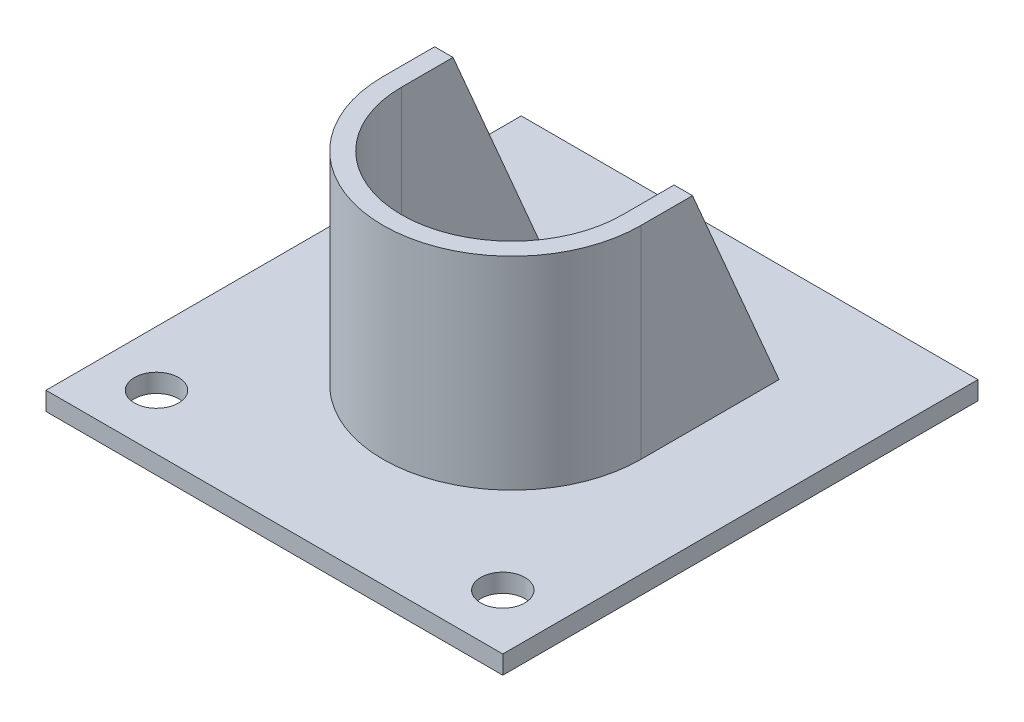
ISO-10303-21;
HEADER;
FILE_DESCRIPTION(('STEP AP214'),'2;1');
FILE_NAME('part.step','',(''),(''),'','','');
FILE_SCHEMA(('AUTOMOTIVE_DESIGN { 1 0 10303 214 1 1 1 1 }'));
ENDSEC;
DATA;
#1=APPLICATION_CONTEXT('core data for automotive mechanical design processes');
#2=APPLICATION_PROTOCOL_DEFINITION('international standard','automotive_design',2000,#1);
#3=PRODUCT_CONTEXT('',#1,'mechanical');
#4=PRODUCT('Part','Part','',(#3));
#5=PRODUCT_RELATED_PRODUCT_CATEGORY('part','',(#4));
#6=PRODUCT_DEFINITION_FORMATION('','',#4);
#7=PRODUCT_DEFINITION_CONTEXT('part definition',#1,'design');
#8=PRODUCT_DEFINITION('design','',#6,#7);
#9=PRODUCT_DEFINITION_SHAPE('','',#8);
#10=(LENGTH_UNIT() NAMED_UNIT(*) SI_UNIT(.MILLI.,.METRE.));
#11=(NAMED_UNIT(*) PLANE_ANGLE_UNIT() SI_UNIT($,.RADIAN.));
#12=(NAMED_UNIT(*) SI_UNIT($,.STERADIAN.) SOLID_ANGLE_UNIT());
#13=UNCERTAINTY_MEASURE_WITH_UNIT(LENGTH_MEASURE(1.E-05),#10,'distance_accuracy_value','');
#14=(GEOMETRIC_REPRESENTATION_CONTEXT(3) GLOBAL_UNCERTAINTY_ASSIGNED_CONTEXT((#13)) GLOBAL_UNIT_ASSIGNED_CONTEXT((#10,
#11,#12)) REPRESENTATION_CONTEXT('',''));
#15=CARTESIAN_POINT('',(0.,0.,0.));
#16=DIRECTION('',(0.,0.,1.));
#17=DIRECTION('',(1.,0.,0.));
#18=AXIS2_PLACEMENT_3D('',#15,#16,#17);
#19=CARTESIAN_POINT('',(35.,5.,-37.5));
#20=DIRECTION('',(0.,-0.392910121106435,0.919576879185273));
#21=DIRECTION('',(0.,-0.919576879185273,-0.392910121106435));
#22=AXIS2_PLACEMENT_3D('',#19,#20,#21);
#23=PLANE('',#22);
#24=DIRECTION('',(-1.,0.,0.));
#25=VECTOR('',#24,1.);
#26=CARTESIAN_POINT('',(35.,5.,-37.5));
#27=LINE('',#26,#25);
#28=CARTESIAN_POINT('',(35.,5.,-37.5));
#29=VERTEX_POINT('',#28);
#30=CARTESIAN_POINT('',(30.,5.,-37.5));
#31=VERTEX_POINT('',#30);
#32=EDGE_CURVE('E176',#29,#31,#27,.T.);
#33=ORIENTED_EDGE('',*,*,#32,.T.);
#34=DIRECTION('',(0.,0.919576879185273,0.392910121106435));
#35=VECTOR('',#34,1.);
#36=CARTESIAN_POINT('',(30.,5.,-37.5));
#37=LINE('',#36,#35);
#38=CARTESIAN_POINT('',(30.,60.,-14.));
#39=VERTEX_POINT('',#38);
#40=EDGE_CURVE('E12',#31,#39,#37,.T.);
#41=ORIENTED_EDGE('',*,*,#40,.T.);
#42=DIRECTION('',(-1.,0.,0.));
#43=VECTOR('',#42,1.);
#44=CARTESIAN_POINT('',(35.,60.,-14.));
#45=LINE('',#44,#43);
#46=CARTESIAN_POINT('',(35.,60.,-14.));
#47=VERTEX_POINT('',#46);
#48=EDGE_CURVE('E162',#47,#39,#45,.T.);
#49=ORIENTED_EDGE('',*,*,#48,.F.);
#50=DIRECTION('',(0.,0.919576879185273,0.392910121106435));
#51=VECTOR('',#50,1.);
#52=CARTESIAN_POINT('',(35.,5.,-37.5));
#53=LINE('',#52,#51);
#54=EDGE_CURVE('E157',#29,#47,#53,.T.);
#55=ORIENTED_EDGE('',*,*,#54,.F.);
#56=EDGE_LOOP('',(#33,#41,#49,#55));
#57=FACE_BOUND('',#56,.T.);
#58=ADVANCED_FACE('F60',(#57),#23,.F.);
#59=CARTESIAN_POINT('',(35.,60.,-14.));
#60=DIRECTION('',(0.,-1.,0.));
#61=DIRECTION('',(0.,0.,-1.));
#62=AXIS2_PLACEMENT_3D('',#59,#60,#61);
#63=PLANE('',#62);
#64=CARTESIAN_POINT('',(0.,60.,0.));
#65=DIRECTION('',(0.,1.,0.));
#66=DIRECTION('',(0.,0.,1.));
#67=AXIS2_PLACEMENT_3D('',#64,#65,#66);
#68=CIRCLE('',#67,35.);
#69=CARTESIAN_POINT('',(-35.,60.,0.));
#70=VERTEX_POINT('',#69);
#71=CARTESIAN_POINT('',(35.,60.,0.));
#72=VERTEX_POINT('',#71);
#73=EDGE_CURVE('E79',#70,#72,#68,.T.);
#74=ORIENTED_EDGE('',*,*,#73,.T.);
#75=DIRECTION('',(0.,0.,1.));
#76=VECTOR('',#75,1.);
#77=CARTESIAN_POINT('',(35.,60.,-14.));
#78=LINE('',#77,#76);
#79=EDGE_CURVE('E146',#47,#72,#78,.T.);
#80=ORIENTED_EDGE('',*,*,#79,.F.);
#81=ORIENTED_EDGE('',*,*,#48,.T.);
#82=DIRECTION('',(0.,0.,-1.));
#83=VECTOR('',#82,1.);
#84=CARTESIAN_POINT('',(30.,60.,0.));
#85=LINE('',#84,#83);
#86=CARTESIAN_POINT('',(30.,60.,0.));
#87=VERTEX_POINT('',#86);
#88=EDGE_CURVE('E243',#87,#39,#85,.T.);
#89=ORIENTED_EDGE('',*,*,#88,.F.);
#90=CARTESIAN_POINT('',(0.,60.,0.));
#91=DIRECTION('',(0.,1.,0.));
#92=DIRECTION('',(0.,0.,1.));
#93=AXIS2_PLACEMENT_3D('',#90,#91,#92);
#94=CIRCLE('',#93,30.);
#95=CARTESIAN_POINT('',(-30.,60.,0.));
#96=VERTEX_POINT('',#95);
#97=EDGE_CURVE('E242',#96,#87,#94,.T.);
#98=ORIENTED_EDGE('',*,*,#97,.F.);
#99=DIRECTION('',(0.,0.,1.));
#100=VECTOR('',#99,1.);
#101=CARTESIAN_POINT('',(-30.,60.,0.));
#102=LINE('',#101,#100);
#103=CARTESIAN_POINT('',(-30.,60.,-14.));
#104=VERTEX_POINT('',#103);
#105=EDGE_CURVE('E229',#104,#96,#102,.T.);
#106=ORIENTED_EDGE('',*,*,#105,.F.);
#107=CARTESIAN_POINT('',(-35.,60.,-14.));
#108=VERTEX_POINT('',#107);
#109=EDGE_CURVE('E161',#104,#108,#45,.T.);
#110=ORIENTED_EDGE('',*,*,#109,.T.);
#111=DIRECTION('',(0.,0.,1.));
#112=VECTOR('',#111,1.);
#113=CARTESIAN_POINT('',(-35.,60.,-14.));
#114=LINE('',#113,#112);
#115=EDGE_CURVE('E147',#108,#70,#114,.T.);
#116=ORIENTED_EDGE('',*,*,#115,.T.);
#117=EDGE_LOOP('',(#74,#80,#81,#89,#98,#106,#110,#116));
#118=FACE_BOUND('',#117,.T.);
#119=ADVANCED_FACE('F144',(#118),#63,.F.);
#120=CARTESIAN_POINT('',(0.,5.,0.));
#121=DIRECTION('',(0.,1.,0.));
#122=DIRECTION('',(0.,0.,1.));
#123=AXIS2_PLACEMENT_3D('',#120,#121,#122);
#124=PLANE('',#123);
#125=DIRECTION('',(0.,0.,-1.));
#126=VECTOR('',#125,1.);
#127=CARTESIAN_POINT('',(35.,5.,-37.5));
#128=LINE('',#127,#126);
#129=CARTESIAN_POINT('',(35.,5.,0.));
#130=VERTEX_POINT('',#129);
#131=EDGE_CURVE('E164',#130,#29,#128,.T.);
#132=ORIENTED_EDGE('',*,*,#131,.F.);
#133=CARTESIAN_POINT('',(0.,5.,0.));
#134=DIRECTION('',(0.,1.,0.));
#135=DIRECTION('',(0.,0.,1.));
#136=AXIS2_PLACEMENT_3D('',#133,#134,#135);
#137=CIRCLE('',#136,35.);
#138=CARTESIAN_POINT('',(-35.,5.,0.));
#139=VERTEX_POINT('',#138);
#140=EDGE_CURVE('E75',#139,#130,#137,.T.);
#141=ORIENTED_EDGE('',*,*,#140,.F.);
#142=DIRECTION('',(0.,0.,-1.));
#143=VECTOR('',#142,1.);
#144=CARTESIAN_POINT('',(-35.,5.,-37.5));
#145=LINE('',#144,#143);
#146=CARTESIAN_POINT('',(-35.,5.,-37.5));
#147=VERTEX_POINT('',#146);
#148=EDGE_CURVE('E166',#139,#147,#145,.T.);
#149=ORIENTED_EDGE('',*,*,#148,.T.);
#150=CARTESIAN_POINT('',(-30.,5.,-37.5));
#151=VERTEX_POINT('',#150);
#152=EDGE_CURVE('E179',#151,#147,#27,.T.);
#153=ORIENTED_EDGE('',*,*,#152,.F.);
#154=DIRECTION('',(0.,0.,-1.));
#155=VECTOR('',#154,1.);
#156=CARTESIAN_POINT('',(-30.,5.,0.));
#157=LINE('',#156,#155);
#158=CARTESIAN_POINT('',(-30.,5.,0.));
#159=VERTEX_POINT('',#158);
#160=EDGE_CURVE('E248',#159,#151,#157,.T.);
#161=ORIENTED_EDGE('',*,*,#160,.F.);
#162=CARTESIAN_POINT('',(0.,5.,0.));
#163=DIRECTION('',(0.,1.,0.));
#164=DIRECTION('',(0.,0.,1.));
#165=AXIS2_PLACEMENT_3D('',#162,#163,#164);
#166=CIRCLE('',#165,30.);
#167=CARTESIAN_POINT('',(30.,5.,0.));
#168=VERTEX_POINT('',#167);
#169=EDGE_CURVE('E256',#168,#159,#166,.F.);
#170=ORIENTED_EDGE('',*,*,#169,.F.);
#171=DIRECTION('',(0.,0.,1.));
#172=VECTOR('',#171,1.);
#173=CARTESIAN_POINT('',(30.,5.,0.));
#174=LINE('',#173,#172);
#175=EDGE_CURVE('E174',#31,#168,#174,.T.);
#176=ORIENTED_EDGE('',*,*,#175,.F.);
#177=ORIENTED_EDGE('',*,*,#32,.F.);
#178=EDGE_LOOP('',(#132,#141,#149,#153,#161,#170,#176,#177));
#179=FACE_BOUND('',#178,.T.);
#180=CARTESIAN_POINT('',(47.,5.,49.5));
#181=DIRECTION('',(0.,1.,0.));
#182=DIRECTION('',(0.,0.,1.));
#183=AXIS2_PLACEMENT_3D('',#180,#181,#182);
#184=CIRCLE('',#183,6.00000000000001);
#185=CARTESIAN_POINT('',(47.,5.,55.5));
#186=VERTEX_POINT('',#185);
#187=EDGE_CURVE('E189',#186,#186,#184,.T.);
#188=ORIENTED_EDGE('',*,*,#187,.F.);
#189=EDGE_LOOP('',(#188));
#190=FACE_BOUND('',#189,.T.);
#191=DIRECTION('',(0.,0.,-1.));
#192=VECTOR('',#191,1.);
#193=CARTESIAN_POINT('',(62.,5.,-64.5));
#194=LINE('',#193,#192);
#195=CARTESIAN_POINT('',(62.,5.,64.5));
#196=VERTEX_POINT('',#195);
#197=CARTESIAN_POINT('',(62.,5.,-64.5));
#198=VERTEX_POINT('',#197);
#199=EDGE_CURVE('E200',#196,#198,#194,.T.);
#200=ORIENTED_EDGE('',*,*,#199,.T.);
#201=DIRECTION('',(-1.,0.,0.));
#202=VECTOR('',#201,1.);
#203=CARTESIAN_POINT('',(-62.,5.,-64.5));
#204=LINE('',#203,#202);
#205=CARTESIAN_POINT('',(-62.,5.,-64.5));
#206=VERTEX_POINT('',#205);
#207=EDGE_CURVE('E205',#198,#206,#204,.T.);
#208=ORIENTED_EDGE('',*,*,#207,.T.);
#209=DIRECTION('',(0.,0.,1.));
#210=VECTOR('',#209,1.);
#211=CARTESIAN_POINT('',(-62.,5.,-64.5));
#212=LINE('',#211,#210);
#213=CARTESIAN_POINT('',(-62.,5.,64.5));
#214=VERTEX_POINT('',#213);
#215=EDGE_CURVE('E202',#206,#214,#212,.T.);
#216=ORIENTED_EDGE('',*,*,#215,.T.);
#217=DIRECTION('',(1.,0.,0.));
#218=VECTOR('',#217,1.);
#219=CARTESIAN_POINT('',(-62.,5.,64.5));
#220=LINE('',#219,#218);
#221=EDGE_CURVE('E210',#214,#196,#220,.T.);
#222=ORIENTED_EDGE('',*,*,#221,.T.);
#223=EDGE_LOOP('',(#200,#208,#216,#222));
#224=FACE_BOUND('',#223,.T.);
#225=CARTESIAN_POINT('',(0.,5.,-49.5));
#226=DIRECTION('',(0.,1.,0.));
#227=DIRECTION('',(0.,0.,1.));
#228=AXIS2_PLACEMENT_3D('',#225,#226,#227);
#229=CIRCLE('',#228,6.);
#230=CARTESIAN_POINT('',(0.,5.,-43.5));
#231=VERTEX_POINT('',#230);
#232=EDGE_CURVE('E195',#231,#231,#229,.T.);
#233=ORIENTED_EDGE('',*,*,#232,.F.);
#234=EDGE_LOOP('',(#233));
#235=FACE_BOUND('',#234,.T.);
#236=CARTESIAN_POINT('',(-47.,5.,49.5));
#237=DIRECTION('',(0.,1.,0.));
#238=DIRECTION('',(0.,0.,1.));
#239=AXIS2_PLACEMENT_3D('',#236,#237,#238);
#240=CIRCLE('',#239,5.99999999999999);
#241=CARTESIAN_POINT('',(-47.,5.,55.5));
#242=VERTEX_POINT('',#241);
#243=EDGE_CURVE('E182',#242,#242,#240,.T.);
#244=ORIENTED_EDGE('',*,*,#243,.F.);
#245=EDGE_LOOP('',(#244));
#246=FACE_BOUND('',#245,.T.);
#247=ADVANCED_FACE('F255',(#179,#190,#224,#235,#246),#124,.T.);
#248=CARTESIAN_POINT('',(0.,0.,0.));
#249=DIRECTION('',(0.,1.,0.));
#250=DIRECTION('',(0.,0.,1.));
#251=AXIS2_PLACEMENT_3D('',#248,#249,#250);
#252=PLANE('',#251);
#253=DIRECTION('',(0.,0.,-1.));
#254=VECTOR('',#253,1.);
#255=CARTESIAN_POINT('',(62.,0.,-64.5));
#256=LINE('',#255,#254);
#257=CARTESIAN_POINT('',(62.,0.,64.5));
#258=VERTEX_POINT('',#257);
#259=CARTESIAN_POINT('',(62.,0.,-64.5));
#260=VERTEX_POINT('',#259);
#261=EDGE_CURVE('E198',#258,#260,#256,.T.);
#262=ORIENTED_EDGE('',*,*,#261,.F.);
#263=DIRECTION('',(1.,0.,0.));
#264=VECTOR('',#263,1.);
#265=CARTESIAN_POINT('',(-62.,0.,64.5));
#266=LINE('',#265,#264);
#267=CARTESIAN_POINT('',(-62.,0.,64.5));
#268=VERTEX_POINT('',#267);
#269=EDGE_CURVE('E201',#268,#258,#266,.T.);
#270=ORIENTED_EDGE('',*,*,#269,.F.);
#271=DIRECTION('',(0.,0.,1.));
#272=VECTOR('',#271,1.);
#273=CARTESIAN_POINT('',(-62.,0.,-64.5));
#274=LINE('',#273,#272);
#275=CARTESIAN_POINT('',(-62.,0.,-64.5));
#276=VERTEX_POINT('',#275);
#277=EDGE_CURVE('E212',#276,#268,#274,.T.);
#278=ORIENTED_EDGE('',*,*,#277,.F.);
#279=DIRECTION('',(-1.,0.,0.));
#280=VECTOR('',#279,1.);
#281=CARTESIAN_POINT('',(-62.,0.,-64.5));
#282=LINE('',#281,#280);
#283=EDGE_CURVE('E215',#260,#276,#282,.T.);
#284=ORIENTED_EDGE('',*,*,#283,.F.);
#285=EDGE_LOOP('',(#262,#270,#278,#284));
#286=FACE_BOUND('',#285,.T.);
#287=CARTESIAN_POINT('',(0.,0.,-49.5));
#288=DIRECTION('',(0.,1.,0.));
#289=DIRECTION('',(0.,0.,1.));
#290=AXIS2_PLACEMENT_3D('',#287,#288,#289);
#291=CIRCLE('',#290,6.);
#292=CARTESIAN_POINT('',(0.,0.,-43.5));
#293=VERTEX_POINT('',#292);
#294=EDGE_CURVE('E186',#293,#293,#291,.T.);
#295=ORIENTED_EDGE('',*,*,#294,.T.);
#296=EDGE_LOOP('',(#295));
#297=FACE_BOUND('',#296,.T.);
#298=CARTESIAN_POINT('',(47.,0.,49.5));
#299=DIRECTION('',(0.,1.,0.));
#300=DIRECTION('',(0.,0.,1.));
#301=AXIS2_PLACEMENT_3D('',#298,#299,#300);
#302=CIRCLE('',#301,6.00000000000001);
#303=CARTESIAN_POINT('',(47.,0.,55.5));
#304=VERTEX_POINT('',#303);
#305=EDGE_CURVE('E184',#304,#304,#302,.T.);
#306=ORIENTED_EDGE('',*,*,#305,.T.);
#307=EDGE_LOOP('',(#306));
#308=FACE_BOUND('',#307,.T.);
#309=CARTESIAN_POINT('',(-47.,0.,49.5));
#310=DIRECTION('',(0.,1.,0.));
#311=DIRECTION('',(0.,0.,1.));
#312=AXIS2_PLACEMENT_3D('',#309,#310,#311);
#313=CIRCLE('',#312,5.99999999999999);
#314=CARTESIAN_POINT('',(-47.,0.,55.5));
#315=VERTEX_POINT('',#314);
#316=EDGE_CURVE('E177',#315,#315,#313,.T.);
#317=ORIENTED_EDGE('',*,*,#316,.T.);
#318=EDGE_LOOP('',(#317));
#319=FACE_BOUND('',#318,.T.);
#320=ADVANCED_FACE('F311',(#286,#297,#308,#319),#252,.F.);
#321=CARTESIAN_POINT('',(62.,5.,-64.5));
#322=DIRECTION('',(-1.,0.,0.));
#323=DIRECTION('',(0.,0.,1.));
#324=AXIS2_PLACEMENT_3D('',#321,#322,#323);
#325=PLANE('',#324);
#326=ORIENTED_EDGE('',*,*,#261,.T.);
#327=DIRECTION('',(0.,-1.,0.));
#328=VECTOR('',#327,1.);
#329=CARTESIAN_POINT('',(62.,5.,-64.5));
#330=LINE('',#329,#328);
#331=EDGE_CURVE('E223',#198,#260,#330,.T.);
#332=ORIENTED_EDGE('',*,*,#331,.F.);
#333=ORIENTED_EDGE('',*,*,#199,.F.);
#334=DIRECTION('',(0.,-1.,0.));
#335=VECTOR('',#334,1.);
#336=CARTESIAN_POINT('',(62.,5.,64.5));
#337=LINE('',#336,#335);
#338=EDGE_CURVE('E207',#196,#258,#337,.T.);
#339=ORIENTED_EDGE('',*,*,#338,.T.);
#340=EDGE_LOOP('',(#326,#332,#333,#339));
#341=FACE_BOUND('',#340,.T.);
#342=ADVANCED_FACE('F56',(#341),#325,.F.);
#343=CARTESIAN_POINT('',(-62.,5.,-64.5));
#344=DIRECTION('',(0.,0.,1.));
#345=DIRECTION('',(1.,0.,0.));
#346=AXIS2_PLACEMENT_3D('',#343,#344,#345);
#347=PLANE('',#346);
#348=ORIENTED_EDGE('',*,*,#283,.T.);
#349=DIRECTION('',(0.,-1.,0.));
#350=VECTOR('',#349,1.);
#351=CARTESIAN_POINT('',(-62.,5.,-64.5));
#352=LINE('',#351,#350);
#353=EDGE_CURVE('E225',#206,#276,#352,.T.);
#354=ORIENTED_EDGE('',*,*,#353,.F.);
#355=ORIENTED_EDGE('',*,*,#207,.F.);
#356=ORIENTED_EDGE('',*,*,#331,.T.);
#357=EDGE_LOOP('',(#348,#354,#355,#356));
#358=FACE_BOUND('',#357,.T.);
#359=ADVANCED_FACE('F325',(#358),#347,.F.);
#360=CARTESIAN_POINT('',(-62.,5.,-64.5));
#361=DIRECTION('',(1.,0.,0.));
#362=DIRECTION('',(0.,0.,-1.));
#363=AXIS2_PLACEMENT_3D('',#360,#361,#362);
#364=PLANE('',#363);
#365=ORIENTED_EDGE('',*,*,#277,.T.);
#366=DIRECTION('',(0.,-1.,0.));
#367=VECTOR('',#366,1.);
#368=CARTESIAN_POINT('',(-62.,5.,64.5));
#369=LINE('',#368,#367);
#370=EDGE_CURVE('E218',#214,#268,#369,.T.);
#371=ORIENTED_EDGE('',*,*,#370,.F.);
#372=ORIENTED_EDGE('',*,*,#215,.F.);
#373=ORIENTED_EDGE('',*,*,#353,.T.);
#374=EDGE_LOOP('',(#365,#371,#372,#373));
#375=FACE_BOUND('',#374,.T.);
#376=ADVANCED_FACE('F317',(#375),#364,.F.);
#377=CARTESIAN_POINT('',(-62.,5.,64.5));
#378=DIRECTION('',(0.,0.,-1.));
#379=DIRECTION('',(-1.,0.,0.));
#380=AXIS2_PLACEMENT_3D('',#377,#378,#379);
#381=PLANE('',#380);
#382=ORIENTED_EDGE('',*,*,#269,.T.);
#383=ORIENTED_EDGE('',*,*,#338,.F.);
#384=ORIENTED_EDGE('',*,*,#221,.F.);
#385=ORIENTED_EDGE('',*,*,#370,.T.);
#386=EDGE_LOOP('',(#382,#383,#384,#385));
#387=FACE_BOUND('',#386,.T.);
#388=ADVANCED_FACE('F310',(#387),#381,.F.);
#389=CARTESIAN_POINT('',(0.,5.,-49.5));
#390=DIRECTION('',(0.,-1.,0.));
#391=DIRECTION('',(0.,0.,-1.));
#392=AXIS2_PLACEMENT_3D('',#389,#390,#391);
#393=CYLINDRICAL_SURFACE('',#392,6.);
#394=ORIENTED_EDGE('',*,*,#232,.T.);
#395=EDGE_LOOP('',(#394));
#396=FACE_BOUND('',#395,.T.);
#397=ORIENTED_EDGE('',*,*,#294,.F.);
#398=EDGE_LOOP('',(#397));
#399=FACE_BOUND('',#398,.T.);
#400=ADVANCED_FACE('F301',(#396,#399),#393,.F.);
#401=CARTESIAN_POINT('',(47.,5.,49.5));
#402=DIRECTION('',(0.,-1.,0.));
#403=DIRECTION('',(0.,0.,-1.));
#404=AXIS2_PLACEMENT_3D('',#401,#402,#403);
#405=CYLINDRICAL_SURFACE('',#404,6.00000000000001);
#406=ORIENTED_EDGE('',*,*,#187,.T.);
#407=EDGE_LOOP('',(#406));
#408=FACE_BOUND('',#407,.T.);
#409=ORIENTED_EDGE('',*,*,#305,.F.);
#410=EDGE_LOOP('',(#409));
#411=FACE_BOUND('',#410,.T.);
#412=ADVANCED_FACE('F299',(#408,#411),#405,.F.);
#413=CARTESIAN_POINT('',(-47.,5.,49.5));
#414=DIRECTION('',(0.,-1.,0.));
#415=DIRECTION('',(0.,0.,-1.));
#416=AXIS2_PLACEMENT_3D('',#413,#414,#415);
#417=CYLINDRICAL_SURFACE('',#416,5.99999999999999);
#418=ORIENTED_EDGE('',*,*,#243,.T.);
#419=EDGE_LOOP('',(#418));
#420=FACE_BOUND('',#419,.T.);
#421=ORIENTED_EDGE('',*,*,#316,.F.);
#422=EDGE_LOOP('',(#421));
#423=FACE_BOUND('',#422,.T.);
#424=ADVANCED_FACE('F294',(#420,#423),#417,.F.);
#425=ORIENTED_EDGE('',*,*,#109,.F.);
#426=DIRECTION('',(0.,-0.919576879185273,-0.392910121106435));
#427=VECTOR('',#426,1.);
#428=CARTESIAN_POINT('',(-30.,5.,-37.5));
#429=LINE('',#428,#427);
#430=EDGE_CURVE('E61',#104,#151,#429,.T.);
#431=ORIENTED_EDGE('',*,*,#430,.T.);
#432=ORIENTED_EDGE('',*,*,#152,.T.);
#433=DIRECTION('',(0.,0.919576879185273,0.392910121106435));
#434=VECTOR('',#433,1.);
#435=CARTESIAN_POINT('',(-35.,5.,-37.5));
#436=LINE('',#435,#434);
#437=EDGE_CURVE('E173',#147,#108,#436,.T.);
#438=ORIENTED_EDGE('',*,*,#437,.T.);
#439=EDGE_LOOP('',(#425,#431,#432,#438));
#440=FACE_BOUND('',#439,.T.);
#441=ADVANCED_FACE('F273',(#440),#23,.F.);
#442=CARTESIAN_POINT('',(35.,0.,0.));
#443=DIRECTION('',(1.,0.,0.));
#444=DIRECTION('',(0.,0.,-1.));
#445=AXIS2_PLACEMENT_3D('',#442,#443,#444);
#446=PLANE('',#445);
#447=DIRECTION('',(0.,1.,0.));
#448=VECTOR('',#447,1.);
#449=CARTESIAN_POINT('',(35.,5.,0.));
#450=LINE('',#449,#448);
#451=EDGE_CURVE('E151',#130,#72,#450,.T.);
#452=ORIENTED_EDGE('',*,*,#451,.F.);
#453=ORIENTED_EDGE('',*,*,#131,.T.);
#454=ORIENTED_EDGE('',*,*,#54,.T.);
#455=ORIENTED_EDGE('',*,*,#79,.T.);
#456=EDGE_LOOP('',(#452,#453,#454,#455));
#457=FACE_BOUND('',#456,.T.);
#458=ADVANCED_FACE('F160',(#457),#446,.T.);
#459=CARTESIAN_POINT('',(-35.,0.,0.));
#460=DIRECTION('',(1.,0.,0.));
#461=DIRECTION('',(0.,0.,-1.));
#462=AXIS2_PLACEMENT_3D('',#459,#460,#461);
#463=PLANE('',#462);
#464=ORIENTED_EDGE('',*,*,#148,.F.);
#465=DIRECTION('',(0.,1.,0.));
#466=VECTOR('',#465,1.);
#467=CARTESIAN_POINT('',(-35.,5.,0.));
#468=LINE('',#467,#466);
#469=EDGE_CURVE('E262',#139,#70,#468,.T.);
#470=ORIENTED_EDGE('',*,*,#469,.T.);
#471=ORIENTED_EDGE('',*,*,#115,.F.);
#472=ORIENTED_EDGE('',*,*,#437,.F.);
#473=EDGE_LOOP('',(#464,#470,#471,#472));
#474=FACE_BOUND('',#473,.T.);
#475=ADVANCED_FACE('F274',(#474),#463,.F.);
#476=CARTESIAN_POINT('',(30.,-85.3119593409422,0.));
#477=DIRECTION('',(1.,0.,0.));
#478=DIRECTION('',(0.,0.,-1.));
#479=AXIS2_PLACEMENT_3D('',#476,#477,#478);
#480=PLANE('',#479);
#481=ORIENTED_EDGE('',*,*,#175,.T.);
#482=DIRECTION('',(0.,1.,0.));
#483=VECTOR('',#482,1.);
#484=CARTESIAN_POINT('',(30.,-85.3119593409422,0.));
#485=LINE('',#484,#483);
#486=EDGE_CURVE('E246',#168,#87,#485,.T.);
#487=ORIENTED_EDGE('',*,*,#486,.T.);
#488=ORIENTED_EDGE('',*,*,#88,.T.);
#489=ORIENTED_EDGE('',*,*,#40,.F.);
#490=EDGE_LOOP('',(#481,#487,#488,#489));
#491=FACE_BOUND('',#490,.T.);
#492=ADVANCED_FACE('F267',(#491),#480,.F.);
#493=CARTESIAN_POINT('',(-30.,-85.3119593409422,0.));
#494=DIRECTION('',(-1.,0.,0.));
#495=DIRECTION('',(0.,0.,1.));
#496=AXIS2_PLACEMENT_3D('',#493,#494,#495);
#497=PLANE('',#496);
#498=ORIENTED_EDGE('',*,*,#105,.T.);
#499=DIRECTION('',(0.,1.,0.));
#500=VECTOR('',#499,1.);
#501=CARTESIAN_POINT('',(-30.,-85.3119593409422,0.));
#502=LINE('',#501,#500);
#503=EDGE_CURVE('E249',#159,#96,#502,.T.);
#504=ORIENTED_EDGE('',*,*,#503,.F.);
#505=ORIENTED_EDGE('',*,*,#160,.T.);
#506=ORIENTED_EDGE('',*,*,#430,.F.);
#507=EDGE_LOOP('',(#498,#504,#505,#506));
#508=FACE_BOUND('',#507,.T.);
#509=ADVANCED_FACE('F275',(#508),#497,.F.);
#510=CARTESIAN_POINT('',(0.,-85.3119593409422,0.));
#511=DIRECTION('',(0.,1.,0.));
#512=DIRECTION('',(0.,0.,1.));
#513=AXIS2_PLACEMENT_3D('',#510,#511,#512);
#514=CYLINDRICAL_SURFACE('',#513,30.);
#515=ORIENTED_EDGE('',*,*,#169,.T.);
#516=ORIENTED_EDGE('',*,*,#503,.T.);
#517=ORIENTED_EDGE('',*,*,#97,.T.);
#518=ORIENTED_EDGE('',*,*,#486,.F.);
#519=EDGE_LOOP('',(#515,#516,#517,#518));
#520=FACE_BOUND('',#519,.T.);
#521=ADVANCED_FACE('F271',(#520),#514,.F.);
#522=CARTESIAN_POINT('',(0.,5.,0.));
#523=DIRECTION('',(0.,1.,0.));
#524=DIRECTION('',(0.,0.,1.));
#525=AXIS2_PLACEMENT_3D('',#522,#523,#524);
#526=CYLINDRICAL_SURFACE('',#525,35.);
#527=ORIENTED_EDGE('',*,*,#73,.F.);
#528=ORIENTED_EDGE('',*,*,#469,.F.);
#529=ORIENTED_EDGE('',*,*,#140,.T.);
#530=ORIENTED_EDGE('',*,*,#451,.T.);
#531=EDGE_LOOP('',(#527,#528,#529,#530));
#532=FACE_BOUND('',#531,.T.);
#533=ADVANCED_FACE('F153',(#532),#526,.T.);
#534=CLOSED_SHELL('',(#58,#119,#247,#320,#342,#359,#376,#388,#400,#412,#424,#441,#458,#475,#492,
#509,#521,#533));
#535=MANIFOLD_SOLID_BREP('B2',#534);
#536=ADVANCED_BREP_SHAPE_REPRESENTATION('',(#18,#535),#14);
#537=SHAPE_DEFINITION_REPRESENTATION(#9,#536);
ENDSEC;
END-ISO-10303-21;
